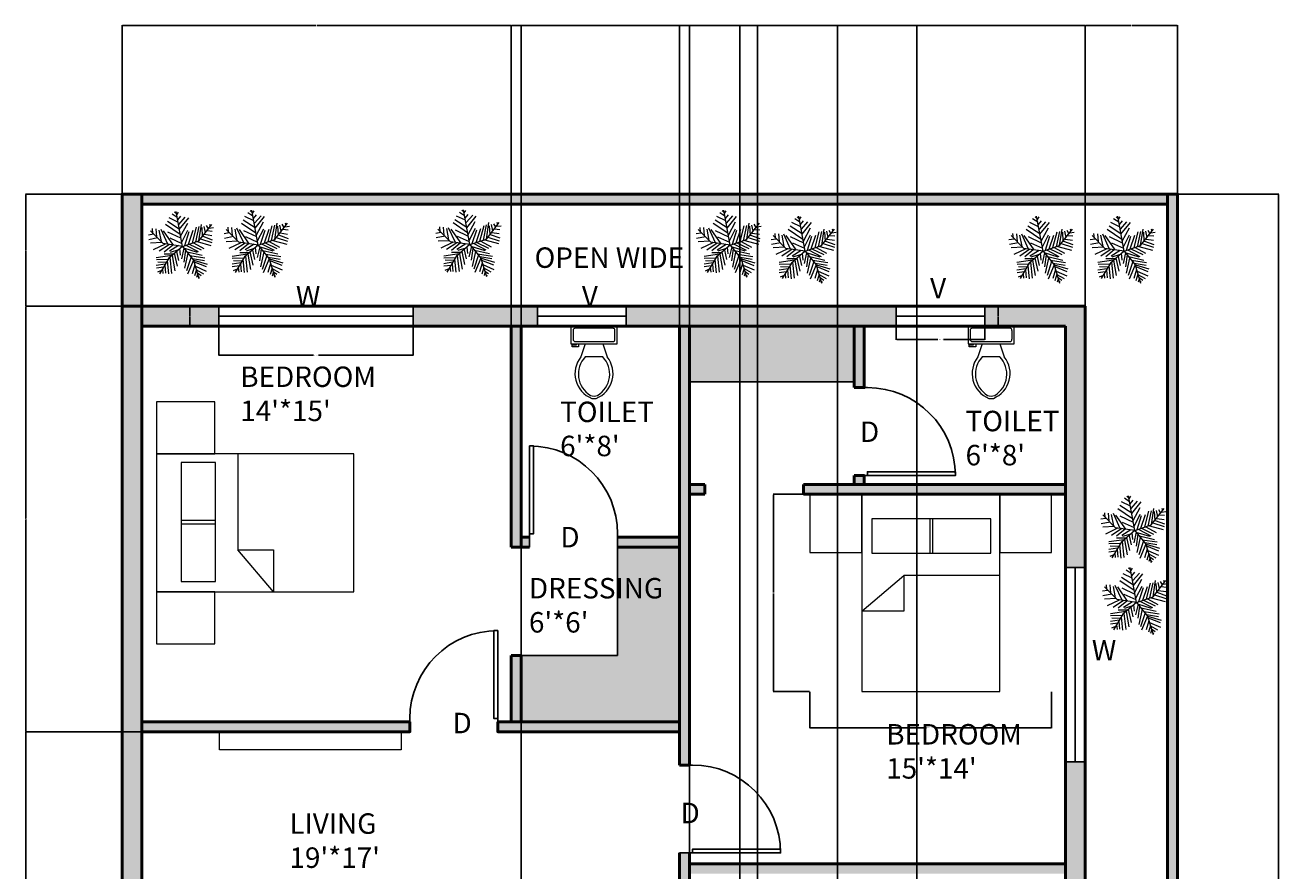
# Model space of a CAD drawing. Units: inches. Extents: x 2024 to 2594, y 643 to 1604.
# Tile 4 of 4: x 2024 to 2594, y 1219 to 1604. Entities that reach past the tile are written whole.
import ezdxf

# ---------------------------------------------------------------- set-up
doc = ezdxf.new("R2010")
doc.units = ezdxf.units.IN
for name, color, linetype, lineweight in [('A-ANNO-DIMS', 2, 'Continuous', 18), ('A-ANNO-TEXT', 7, 'Continuous', 18), ('A-AREA-IDEN', 7, 'Continuous', 25), ('A-CASE-PATT', 54, 'Continuous', 13), ('A-FLOR-CASE', 30, 'Continuous', 25), ('A-FLOR-FIXT', 8, 'Continuous', 18), ('A-WALL-PATT', 50, 'Continuous', 13), ('C-PROP', 7, 'Continuous', 35), ('DOOR', 240, 'Continuous', 25), ('FUR', 212, 'Continuous', 18), ('TREE', 102, 'Continuous', 18), ('WALL', 50, 'Continuous', 50), ('WIN', 140, 'Continuous', 25)]:
    doc.layers.add(name, color=color, linetype=linetype, lineweight=lineweight)
doc.styles.get("Standard").update_dxf_attribs({"font": 'arial.ttf'})
doc.dimstyles.get("Standard").update_dxf_attribs({"dimtxt": 0.18, "dimasz": 0.18, "dimexe": 0.18, "dimexo": 0.0625, "dimgap": 0.09, "dimtad": 0, "dimtih": 1, "dimtoh": 1, "dimdec": 4, "dimzin": 0, "dimdsep": 46, "dimtxsty": 'Standard', "dimcen": 0.09, "dimadec": 0, "dimazin": 0, "dimtfac": 1, "dimtdec": 4, "dimtofl": 0, "dimtmove": 0, "dimatfit": 3, "dimfxl": 1, "dimtolj": 1, "dimtzin": 0, "dimarcsym": 0})

# ---------------------------------------------------------------- blocks, each defined once
blk = doc.blocks.new('*U2')
for p, q in [((0, 0), (0, -6)), ((40, 0), (40, -6))]:
    blk.add_line(p, q)
blk.add_lwpolyline([(0, 0), (0, 40), (1.75, 40), (1.75, 0)], close=True)
blk.add_arc((0, 0), 40, 0, 90)
blk = doc.blocks.new('*U4')
for p, q in [((9.5, -6), (9.5, -2)), ((-10, -8.5), (-8, -8.5)), ((-10, -9.5), (-10, -8.5)), ((-7, -9.5), (-10, -9.5)), ((-8, -8.5), (-8, -8)), ((-7, -8), (-7, -9.5)), ((-4, -8), (-6, -14)), ((4, -8), (6, -14)), ((4, -14), (-4, -14))]:
    blk.add_line(p, q)
blk.add_lwpolyline([(10.5, -8), (10.5, 0), (-10.5, 0), (-10.5, -8)], close=True)
for points in [[(-9.5, -2), (-9.5, -6)], [(8.5, -1), (-8.5, -1)], [(-8.5, -7), (8.5, -7)]]:
    blk.add_lwpolyline(points)
for centre, radius, start, end in [((-8.62, -1.88), 0.884, 81.8699, 188.1301), ((8.62, -1.88), 0.884, 351.8699, 98.1301), ((-8.62, -6.12), 0.884, 171.8699, 278.1301), ((8.62, -6.12), 0.884, 261.8699, 8.1301), ((3.52, -21.58), 12.17, 141.4691, 247.9714), ((4.2, -21.82), 11.33, 136.3677, 238.9468), ((-3.52, -21.58), 12.17, 292.0284, 38.5307), ((-4.2, -21.82), 11.33, 301.053, 43.6321), ((0, -27.88), 4, 245.7318, 294.2682), ((0, -29), 4, 254.8605, 285.1395)]:
    blk.add_arc(centre, radius, start, end)
blk = doc.blocks.new('*U6')
for p, q in [((-7.288, 39.707), (-21.778, 46.673)), ((-8.737, 47.138), (-17.069, 52.711)), ((-10.186, 53.64), (-13.084, 55.962)), ((0, 0), (-10.5, 57)), ((-9.099, 51.782), (-6.563, 55.962)), ((-7.65, 43.423), (-2.578, 49.46)), ((-5.839, 35.992), (4.667, 48.067)), ((-5.114, 27.632), (10.463, 46.673)), ((-31.5, 4.5), (-52.5, 25.5)), ((-48.585, 21.131), (-49.309, 29.026)), ((-43.513, 28.561), (-42.427, 15.558)), ((-38.442, 26.239), (-34.819, 7.663)), ((-35.544, 28.097), (-24.314, 3.947)), ((-14.533, 2.09), (-30.834, 25.31)), ((-3.665, 19.273), (-27.574, 35.527)), ((-5.114, 28.097), (-24.676, 40.636)), ((-24.314, 23.917), (-2.941, 13.7)), ((-2.941, 16.486), (8.652, 37.85)), ((-1.129, 6.734), (9.014, 26.704)), ((3.942, 1.625), (11.187, 24.381)), ((10.101, 3.483), (17.708, 26.239)), ((16.259, 5.805), (23.142, 31.348)), ((22.055, 7.198), (27.489, 32.277)), ((27, 9), (48, 36)), ((27.127, 9.056), (31.112, 35.992)), ((31.836, 30.883), (32.561, 16.486)), ((35.096, 32.741), (37.27, 22.524)), ((38.719, 34.134), (41.979, 28.561)), ((40.53, 25.775), (48.862, 24.846)), ((43.791, 29.954), (51.036, 30.883)), ((44.153, 36.456), (45.239, 32.741)), ((-47.498, 19.737), (-55.83, 18.344)), ((-40.615, 13.7), (-55.105, 10.913)), ((-33.37, 6.269), (-52.207, 5.34)), ((-28.299, 3.483), (-47.86, -5.805)), ((-21.416, 3.018), (-38.079, -8.128)), ((0, 0), (-31.5, 4.5)), ((-15.982, 2.09), (-30.11, -9.521)), ((0, 0), (-22.5, -19.5)), ((-6.563, 1.161), (-21.416, -8.128)), ((-20.691, 13.7), (-1.129, 4.876)), ((0, 0), (27, 9)), ((0, 0), (18, -22.5)), ((6.478, 1.625), (26.04, -8.592)), ((11.187, 3.483), (30.749, -5.805)), ((18.07, 5.805), (35.096, -3.483)), ((24.229, 7.663), (46.688, 1.625)), ((29.662, 12.307), (48.137, 6.269)), ((33.285, 16.486), (48.862, 10.913)), ((36.183, 19.737), (48.137, 17.88)), ((-17.431, -15.094), (-42.789, -18.809)), ((-22.5, -19.5), (-37.5, -45)), ((-15.257, -12.772), (-30.11, -12.772)), ((-20.691, -18.345), (-17.793, -44.352)), ((-6.563, -5.805), (-19.967, -9.985)), ((-17.069, -15.094), (-12.721, -40.172)), ((-13.446, -11.378), (-8.737, -32.741)), ((-9.461, -8.592), (-6.201, -23.453)), ((-4.752, -3.483), (-3.665, -14.629)), ((2.493, -3.019), (-1.491, -20.202)), ((1.769, -2.555), (24.229, -9.521)), ((5.029, -6.27), (2.131, -25.775)), ((9.014, -11.378), (3.58, -35.992)), ((14.085, -16.951), (6.478, -40.172)), ((7.565, -9.056), (32.198, -14.629)), ((12.274, -15.094), (36.907, -18.809)), ((16.259, -19.738), (36.183, -22.989)), ((-28.299, -29.026), (-42.789, -31.348)), ((-24.314, -21.596), (-42.427, -22.06)), ((-30.834, -34.135), (-42.427, -35.528)), ((-34.457, -39.708), (-40.978, -42.494)), ((-26.849, -26.24), (-40.253, -25.775)), ((-32.646, -36.921), (-31.921, -44.352)), ((-29.023, -30.884), (-27.936, -43.887)), ((-25.038, -23.918), (-22.865, -45.281)), ((18.07, -22.524), (8.289, -45.745)), ((20.244, -30.419), (15.897, -44.816)), ((18, -22.5), (27, -52.5)), ((18.433, -22.524), (40.53, -29.026)), ((19.157, -25.311), (38.719, -33.206)), ((22.78, -37.85), (19.519, -48.532)), ((21.331, -32.741), (39.081, -40.636)), ((22.78, -38.314), (34.372, -44.816)), ((24.591, -45.745), (23.142, -50.854)), ((24.591, -43.423), (30.749, -47.603)), ((26.764, -49.925), (28.213, -50.854))]:
    blk.add_line(p, q)
blk = doc.blocks.new('BED-DOUBLE-WITH-NIGHTSTANDS')
for p, q in [((36.91, 86.39), (36.91, 42.72)), ((36.91, 42.72), (53.2, 42.72)), ((53.2, 23.62), (36.91, 42.72)), ((53.2, 42.72), (53.2, 23.62))]:
    blk.add_line(p, q)
for points in [[(0, 86.39), (26.45, 86.39), (26.45, 110.01), (0, 110.01)], [(0, 23.62), (89.75, 23.62), (89.75, 86.39), (0, 86.39)], [(11.14, 54.55), (26.84, 54.55), (26.84, 82.37), (11.14, 82.37)], [(11.14, 28.22), (26.84, 28.22), (26.84, 56.03), (11.14, 56.03)], [(0, 0), (26.45, 0), (26.45, 23.62), (0, 23.62)]]:
    blk.add_lwpolyline(points, close=True)
blk = doc.blocks.new('WINDOW-EXTERIOR')
blk.add_line((4.5, 0), (4.5, 88.37))
blk.add_lwpolyline([(0, 0), (9, 0), (9, 88.37), (0, 88.37)], close=True)
blk = doc.blocks.new('VENT-TOILET')
blk.add_line((0, 4.5), (40.27, 4.5))
blk.add_lwpolyline([(0, 0), (40.27, 0), (40.27, 9), (0, 9)], close=True)
blk = doc.blocks.new('*D17')
at = {"layer": 'A-ANNO-DIMS', "color": 0, "lineweight": -2, "transparency": 16777216}
for p, q in [((2112.29, 1466.87), (2112.29, 1453.5)), ((2200.66, 1466.87), (2200.66, 1453.5)), ((2112.47, 1453.68), (2155.36, 1453.68)), ((2200.48, 1453.68), (2157.59, 1453.68))]:
    blk.add_line(p, q, dxfattribs=at)
at = {"layer": 'A-ANNO-DIMS', "color": 0, "lineweight": 100, "transparency": 16777216}
for points in [[(2112.47, 1453.71), (2112.47, 1453.65), (2112.29, 1453.68)], [(2200.48, 1453.71), (2200.48, 1453.65), (2200.66, 1453.68)]]:
    blk.add_solid(points, dxfattribs=at)
at = {"layer": 'Defpoints', "color": 0, "lineweight": 100, "transparency": 16777216}
for p in [(2112.29, 1466.93), (2200.66, 1466.93), (2200.66, 1453.68)]:
    blk.add_point(p, dxfattribs=at)
at = {"layer": 'A-ANNO-DIMS', "color": 0, "transparency": 16777216, "insert": (2156.48, 1453.68), "char_height": 0.18, "attachment_point": 5}
blk.add_mtext('\\A1;WINDOW 88 TYP.', dxfattribs=at)
blk = doc.blocks.new('*D18')
at = {"layer": 'A-ANNO-DIMS', "color": 0, "lineweight": -2, "transparency": 16777216}
for p, q in [((2112.23, 1475.93), (2098.86, 1475.93)), ((2099.04, 1475.75), (2099.04, 1471.61)), ((2099.04, 1467.11), (2099.04, 1471.25)), ((2112.23, 1466.93), (2098.86, 1466.93))]:
    blk.add_line(p, q, dxfattribs=at)
at = {"layer": 'A-ANNO-DIMS', "color": 0, "lineweight": 100, "transparency": 16777216}
for points in [[(2099.01, 1475.75), (2099.07, 1475.75), (2099.04, 1475.93)], [(2099.01, 1467.11), (2099.07, 1467.11), (2099.04, 1466.93)]]:
    blk.add_solid(points, dxfattribs=at)
at = {"layer": 'Defpoints', "color": 0, "lineweight": 100, "transparency": 16777216}
for p in [(2112.29, 1475.93), (2099.04, 1466.93), (2112.29, 1466.93)]:
    blk.add_point(p, dxfattribs=at)
at = {"layer": 'A-ANNO-DIMS', "color": 0, "transparency": 16777216, "insert": (2099.04, 1471.43), "char_height": 0.18, "attachment_point": 5}
blk.add_mtext('\\A1;9 TYP.', dxfattribs=at)
blk = doc.blocks.new('*D19')
at = {"layer": 'A-ANNO-DIMS', "color": 0, "lineweight": -2, "transparency": 16777216}
for p, q in [((2381.02, 1300.62), (2381.02, 1284)), ((2491.03, 1300.62), (2491.03, 1284)), ((2381.2, 1284.18), (2434.08, 1284.18)), ((2490.85, 1284.18), (2437.96, 1284.18))]:
    blk.add_line(p, q, dxfattribs=at)
at = {"layer": 'A-ANNO-DIMS', "color": 0, "lineweight": 100, "transparency": 16777216}
for points in [[(2381.2, 1284.21), (2381.2, 1284.15), (2381.02, 1284.18)], [(2490.85, 1284.21), (2490.85, 1284.15), (2491.03, 1284.18)]]:
    blk.add_solid(points, dxfattribs=at)
at = {"layer": 'Defpoints', "color": 0, "lineweight": 100, "transparency": 16777216}
for p in [(2381.02, 1300.68), (2491.03, 1300.68), (2491.03, 1284.18)]:
    blk.add_point(p, dxfattribs=at)
at = {"layer": 'A-ANNO-DIMS', "color": 0, "transparency": 16777216, "insert": (2436.02, 1284.18), "char_height": 0.18, "attachment_point": 5}
blk.add_mtext('\\A1;BED & NIGHTSTANDS 110 TYP.', dxfattribs=at)
blk = doc.blocks.new('*D20')
at = {"layer": 'A-ANNO-DIMS', "color": 0, "lineweight": -2, "transparency": 16777216}
for p, q in [((2380.95, 1390.43), (2364.33, 1390.43)), ((2364.51, 1390.25), (2364.51, 1345.74)), ((2364.51, 1300.86), (2364.51, 1345.37)), ((2380.95, 1300.68), (2364.33, 1300.68))]:
    blk.add_line(p, q, dxfattribs=at)
at = {"layer": 'A-ANNO-DIMS', "color": 0, "lineweight": 100, "transparency": 16777216}
for points in [[(2364.48, 1390.25), (2364.54, 1390.25), (2364.51, 1390.43)], [(2364.48, 1300.86), (2364.54, 1300.86), (2364.51, 1300.68)]]:
    blk.add_solid(points, dxfattribs=at)
at = {"layer": 'Defpoints', "color": 0, "lineweight": 100, "transparency": 16777216}
for p in [(2381.02, 1390.43), (2364.51, 1300.68), (2381.02, 1300.68)]:
    blk.add_point(p, dxfattribs=at)
at = {"layer": 'A-ANNO-DIMS', "color": 0, "transparency": 16777216, "insert": (2364.51, 1345.56), "char_height": 0.18, "attachment_point": 5}
blk.add_mtext('\\A1;90 TYP.', dxfattribs=at)
blk = doc.blocks.new('*D23')
at = {"layer": 'A-ANNO-DIMS', "color": 0, "lineweight": -2, "transparency": 16777216}
for p, q in [((2420.38, 1466.87), (2420.38, 1460.71)), ((2460.65, 1466.87), (2460.65, 1460.71)), ((2420.56, 1460.89), (2439.25, 1460.89)), ((2460.47, 1460.89), (2441.78, 1460.89))]:
    blk.add_line(p, q, dxfattribs=at)
at = {"layer": 'A-ANNO-DIMS', "color": 0, "lineweight": 100, "transparency": 16777216}
for points in [[(2420.56, 1460.92), (2420.56, 1460.86), (2420.38, 1460.89)], [(2460.47, 1460.92), (2460.47, 1460.86), (2460.65, 1460.89)]]:
    blk.add_solid(points, dxfattribs=at)
at = {"layer": 'Defpoints', "color": 0, "lineweight": 100, "transparency": 16777216}
for p in [(2420.38, 1466.93), (2460.65, 1466.93), (2460.65, 1460.89)]:
    blk.add_point(p, dxfattribs=at)
at = {"layer": 'A-ANNO-DIMS', "color": 0, "transparency": 16777216, "insert": (2440.52, 1460.89), "char_height": 0.18, "attachment_point": 5}
blk.add_mtext('\\A1;BATH VENT 40 TYP.', dxfattribs=at)
blk = doc.blocks.new('*D24')
at = {"layer": 'A-ANNO-DIMS', "color": 0, "lineweight": -2, "transparency": 16777216}
for p, q in [((2460.72, 1475.93), (2466.87, 1475.93)), ((2466.69, 1475.75), (2466.69, 1471.61)), ((2466.69, 1467.11), (2466.69, 1471.25)), ((2460.72, 1466.93), (2466.87, 1466.93))]:
    blk.add_line(p, q, dxfattribs=at)
at = {"layer": 'A-ANNO-DIMS', "color": 0, "lineweight": 100, "transparency": 16777216}
for points in [[(2466.66, 1475.75), (2466.72, 1475.75), (2466.69, 1475.93)], [(2466.66, 1467.11), (2466.72, 1467.11), (2466.69, 1466.93)]]:
    blk.add_solid(points, dxfattribs=at)
at = {"layer": 'Defpoints', "color": 0, "lineweight": 100, "transparency": 16777216}
for p in [(2460.65, 1475.93), (2466.69, 1475.93), (2460.65, 1466.93)]:
    blk.add_point(p, dxfattribs=at)
at = {"layer": 'A-ANNO-DIMS', "color": 0, "transparency": 16777216, "insert": (2466.69, 1471.43), "char_height": 0.18, "attachment_point": 5}
blk.add_mtext('\\A1;9 TYP.', dxfattribs=at)
blk = doc.blocks.new('*D26')
at = {"layer": 'A-ANNO-DIMS', "color": 0, "lineweight": -2, "transparency": 16777216}
for p, q in [((2548.34, 1526.93), (2594.37, 1526.93)), ((2594.19, 1526.75), (2594.19, 1107.11)), ((2594.19, 687.11), (2594.19, 1106.75)), ((2548.34, 686.93), (2594.37, 686.93))]:
    blk.add_line(p, q, dxfattribs=at)
at = {"layer": 'A-ANNO-DIMS', "color": 0, "lineweight": 100, "transparency": 16777216}
for points in [[(2594.16, 1526.75), (2594.22, 1526.75), (2594.19, 1526.93)], [(2594.16, 687.11), (2594.22, 687.11), (2594.19, 686.93)]]:
    blk.add_solid(points, dxfattribs=at)
at = {"layer": 'Defpoints', "color": 0, "lineweight": 100, "transparency": 16777216}
for p in [(2548.27, 1526.93), (2594.19, 1526.93), (2548.27, 686.93)]:
    blk.add_point(p, dxfattribs=at)
at = {"layer": 'A-ANNO-DIMS', "color": 0, "transparency": 16777216, "insert": (2594.19, 1106.93), "char_height": 0.18, "attachment_point": 5}
blk.add_mtext('\\A1;840', dxfattribs=at)
blk = doc.blocks.new('*D27')
at = {"layer": 'A-ANNO-DIMS', "color": 0, "lineweight": -2, "transparency": 16777216}
for p, q in [((2068.27, 1475.99), (2068.27, 1603.82)), ((2068.45, 1603.64), (2156.49, 1603.64)), ((2245.09, 1603.64), (2157.05, 1603.64)), ((2245.27, 1466.99), (2245.27, 1603.82))]:
    blk.add_line(p, q, dxfattribs=at)
at = {"layer": 'A-ANNO-DIMS', "color": 0, "lineweight": 100, "transparency": 16777216}
for points in [[(2068.45, 1603.67), (2068.45, 1603.61), (2068.27, 1603.64)], [(2245.09, 1603.67), (2245.09, 1603.61), (2245.27, 1603.64)]]:
    blk.add_solid(points, dxfattribs=at)
at = {"layer": 'Defpoints', "color": 0, "lineweight": 100, "transparency": 16777216}
for p in [(2245.27, 1603.64), (2068.27, 1475.93), (2245.27, 1466.93)]:
    blk.add_point(p, dxfattribs=at)
at = {"layer": 'A-ANNO-DIMS', "color": 0, "transparency": 16777216, "insert": (2156.77, 1603.64), "char_height": 0.18, "attachment_point": 5}
blk.add_mtext('\\A1;177', dxfattribs=at)
blk = doc.blocks.new('*D28')
at = {"layer": 'A-ANNO-DIMS', "color": 0, "lineweight": -2, "transparency": 16777216}
for p, q in [((2245.27, 1466.99), (2245.27, 1603.82)), ((2245.45, 1603.64), (2283.2, 1603.64)), ((2321.59, 1603.64), (2283.85, 1603.64)), ((2321.77, 1466.99), (2321.77, 1603.82))]:
    blk.add_line(p, q, dxfattribs=at)
at = {"layer": 'A-ANNO-DIMS', "color": 0, "lineweight": 100, "transparency": 16777216}
for points in [[(2245.45, 1603.67), (2245.45, 1603.61), (2245.27, 1603.64)], [(2321.59, 1603.67), (2321.59, 1603.61), (2321.77, 1603.64)]]:
    blk.add_solid(points, dxfattribs=at)
at = {"layer": 'Defpoints', "color": 0, "lineweight": 100, "transparency": 16777216}
for p in [(2321.77, 1603.64), (2245.27, 1466.93), (2321.77, 1466.93)]:
    blk.add_point(p, dxfattribs=at)
at = {"layer": 'A-ANNO-DIMS', "color": 0, "transparency": 16777216, "insert": (2283.52, 1603.64), "char_height": 0.18, "attachment_point": 5}
blk.add_mtext('\\A1;76.5', dxfattribs=at)
blk = doc.blocks.new('*D29')
at = {"layer": 'A-ANNO-DIMS', "color": 0, "lineweight": -2, "transparency": 16777216}
for p, q in [((2321.77, 1466.99), (2321.77, 1603.82)), ((2321.95, 1603.64), (2413.64, 1603.64)), ((2506.09, 1603.64), (2414.41, 1603.64)), ((2506.27, 1475.99), (2506.27, 1603.82))]:
    blk.add_line(p, q, dxfattribs=at)
at = {"layer": 'A-ANNO-DIMS', "color": 0, "lineweight": 100, "transparency": 16777216}
for points in [[(2321.95, 1603.67), (2321.95, 1603.61), (2321.77, 1603.64)], [(2506.09, 1603.67), (2506.09, 1603.61), (2506.27, 1603.64)]]:
    blk.add_solid(points, dxfattribs=at)
at = {"layer": 'Defpoints', "color": 0, "lineweight": 100, "transparency": 16777216}
for p in [(2506.27, 1603.64), (2506.27, 1475.93), (2321.77, 1466.93)]:
    blk.add_point(p, dxfattribs=at)
at = {"layer": 'A-ANNO-DIMS', "color": 0, "transparency": 16777216, "insert": (2414.02, 1603.64), "char_height": 0.18, "attachment_point": 5}
blk.add_mtext('\\A1;184.5', dxfattribs=at)
blk = doc.blocks.new('*D30')
at = {"layer": 'A-ANNO-DIMS', "color": 0, "lineweight": -2, "transparency": 16777216}
for p, q in [((2506.27, 1475.99), (2506.27, 1603.82)), ((2506.45, 1603.64), (2527.05, 1603.64)), ((2548.09, 1603.64), (2527.49, 1603.64)), ((2548.27, 1526.99), (2548.27, 1603.82))]:
    blk.add_line(p, q, dxfattribs=at)
at = {"layer": 'A-ANNO-DIMS', "color": 0, "lineweight": 100, "transparency": 16777216}
for points in [[(2506.45, 1603.67), (2506.45, 1603.61), (2506.27, 1603.64)], [(2548.09, 1603.67), (2548.09, 1603.61), (2548.27, 1603.64)]]:
    blk.add_solid(points, dxfattribs=at)
at = {"layer": 'Defpoints', "color": 0, "lineweight": 100, "transparency": 16777216}
for p in [(2548.27, 1603.64), (2548.27, 1526.93), (2506.27, 1475.93)]:
    blk.add_point(p, dxfattribs=at)
at = {"layer": 'A-ANNO-DIMS', "color": 0, "transparency": 16777216, "insert": (2527.27, 1603.64), "char_height": 0.18, "attachment_point": 5}
blk.add_mtext('\\A1;42', dxfattribs=at)
blk = doc.blocks.new('*D34')
at = {"layer": 'A-ANNO-DIMS', "color": 0, "lineweight": -2, "transparency": 16777216}
for p, q in [((2077.21, 1282.43), (2024.29, 1282.43)), ((2024.47, 1282.25), (2024.47, 1178.36)), ((2024.47, 1074.1), (2024.47, 1177.99)), ((2077.21, 1073.92), (2024.29, 1073.92))]:
    blk.add_line(p, q, dxfattribs=at)
at = {"layer": 'A-ANNO-DIMS', "color": 0, "lineweight": 100, "transparency": 16777216}
for points in [[(2024.44, 1282.25), (2024.5, 1282.25), (2024.47, 1282.43)], [(2024.44, 1074.1), (2024.5, 1074.1), (2024.47, 1073.92)]]:
    blk.add_solid(points, dxfattribs=at)
at = {"layer": 'Defpoints', "color": 0, "lineweight": 100, "transparency": 16777216}
for p in [(2024.47, 1282.43), (2077.27, 1282.43), (2077.27, 1073.92)]:
    blk.add_point(p, dxfattribs=at)
at = {"layer": 'A-ANNO-DIMS', "color": 0, "transparency": 16777216, "insert": (2024.47, 1178.18), "char_height": 0.18, "attachment_point": 5}
blk.add_mtext('\\A1;208.5', dxfattribs=at)
blk = doc.blocks.new('*D35')
at = {"layer": 'A-ANNO-DIMS', "color": 0, "lineweight": -2, "transparency": 16777216}
for p, q in [((2068.21, 1475.93), (2024.29, 1475.93)), ((2024.47, 1475.75), (2024.47, 1379.36)), ((2024.47, 1282.61), (2024.47, 1379)), ((2077.21, 1282.43), (2024.29, 1282.43))]:
    blk.add_line(p, q, dxfattribs=at)
at = {"layer": 'A-ANNO-DIMS', "color": 0, "lineweight": 100, "transparency": 16777216}
for points in [[(2024.44, 1475.75), (2024.5, 1475.75), (2024.47, 1475.93)], [(2024.44, 1282.61), (2024.5, 1282.61), (2024.47, 1282.43)]]:
    blk.add_solid(points, dxfattribs=at)
at = {"layer": 'Defpoints', "color": 0, "lineweight": 100, "transparency": 16777216}
for p in [(2024.47, 1475.93), (2068.27, 1475.93), (2077.27, 1282.43)]:
    blk.add_point(p, dxfattribs=at)
at = {"layer": 'A-ANNO-DIMS', "color": 0, "transparency": 16777216, "insert": (2024.47, 1379.18), "char_height": 0.18, "attachment_point": 5}
blk.add_mtext('\\A1;193.5', dxfattribs=at)
blk = doc.blocks.new('*D36')
at = {"layer": 'A-ANNO-DIMS', "color": 0, "lineweight": -2, "transparency": 16777216}
for p, q in [((2068.21, 1526.93), (2024.29, 1526.93)), ((2024.47, 1526.75), (2024.47, 1501.61)), ((2024.47, 1476.11), (2024.47, 1501.25)), ((2068.21, 1475.93), (2024.29, 1475.93))]:
    blk.add_line(p, q, dxfattribs=at)
at = {"layer": 'A-ANNO-DIMS', "color": 0, "lineweight": 100, "transparency": 16777216}
for points in [[(2024.44, 1526.75), (2024.5, 1526.75), (2024.47, 1526.93)], [(2024.44, 1476.11), (2024.5, 1476.11), (2024.47, 1475.93)]]:
    blk.add_solid(points, dxfattribs=at)
at = {"layer": 'Defpoints', "color": 0, "lineweight": 100, "transparency": 16777216}
for p in [(2024.47, 1526.93), (2068.27, 1526.93), (2068.27, 1475.93)]:
    blk.add_point(p, dxfattribs=at)
at = {"layer": 'A-ANNO-DIMS', "color": 0, "transparency": 16777216, "insert": (2024.47, 1501.43), "char_height": 0.18, "attachment_point": 5}
blk.add_mtext('\\A1;51', dxfattribs=at)
blk = doc.blocks.new('*D37')
at = {"layer": 'A-ANNO-DIMS', "color": 0, "lineweight": -2, "transparency": 16777216}
for p, q in [((2326.27, 1217.99), (2326.27, 1603.82)), ((2326.45, 1603.64), (2359.59, 1603.64)), ((2393.52, 1603.64), (2360.38, 1603.64)), ((2393.7, 1214.56), (2393.7, 1603.82))]:
    blk.add_line(p, q, dxfattribs=at)
at = {"layer": 'A-ANNO-DIMS', "color": 0, "lineweight": 100, "transparency": 16777216}
for points in [[(2326.45, 1603.67), (2326.45, 1603.61), (2326.27, 1603.64)], [(2393.52, 1603.67), (2393.52, 1603.61), (2393.7, 1603.64)]]:
    blk.add_solid(points, dxfattribs=at)
at = {"layer": 'Defpoints', "color": 0, "lineweight": 100, "transparency": 16777216}
for p in [(2393.7, 1603.64), (2326.27, 1217.93), (2393.7, 1214.5)]:
    blk.add_point(p, dxfattribs=at)
at = {"layer": 'A-ANNO-DIMS', "color": 0, "transparency": 16777216, "insert": (2359.99, 1603.64), "char_height": 0.18, "attachment_point": 5}
blk.add_mtext('\\A1;67.43', dxfattribs=at)
blk = doc.blocks.new('*D38')
at = {"layer": 'A-ANNO-DIMS', "color": 0, "lineweight": -2, "transparency": 16777216}
for p, q in [((2393.7, 1214.56), (2393.7, 1603.82)), ((2393.88, 1603.64), (2411.26, 1603.64)), ((2429.57, 1603.64), (2412.19, 1603.64)), ((2429.75, 1214.56), (2429.75, 1603.82))]:
    blk.add_line(p, q, dxfattribs=at)
at = {"layer": 'A-ANNO-DIMS', "color": 0, "lineweight": 100, "transparency": 16777216}
for points in [[(2393.88, 1603.67), (2393.88, 1603.61), (2393.7, 1603.64)], [(2429.57, 1603.67), (2429.57, 1603.61), (2429.75, 1603.64)]]:
    blk.add_solid(points, dxfattribs=at)
at = {"layer": 'Defpoints', "color": 0, "lineweight": 100, "transparency": 16777216}
for p in [(2429.75, 1603.64), (2393.7, 1214.5), (2429.75, 1214.5)]:
    blk.add_point(p, dxfattribs=at)
at = {"layer": 'A-ANNO-DIMS', "color": 0, "transparency": 16777216, "insert": (2411.73, 1603.64), "char_height": 0.18, "attachment_point": 5}
blk.add_mtext('\\A1;36.046', dxfattribs=at)
blk = doc.blocks.new('*D48')
at = {"layer": 'A-ANNO-DIMS', "color": 0, "lineweight": -2, "transparency": 16777216}
for p, q in [((2249.77, 819.02), (2249.77, 1603.82)), ((2249.95, 1603.64), (2299.2, 1603.64)), ((2349.09, 1603.64), (2299.85, 1603.64)), ((2349.27, 860.99), (2349.27, 1603.82))]:
    blk.add_line(p, q, dxfattribs=at)
at = {"layer": 'A-ANNO-DIMS', "color": 0, "lineweight": 100, "transparency": 16777216}
for points in [[(2249.95, 1603.67), (2249.95, 1603.61), (2249.77, 1603.64)], [(2349.09, 1603.67), (2349.09, 1603.61), (2349.27, 1603.64)]]:
    blk.add_solid(points, dxfattribs=at)
at = {"layer": 'Defpoints', "color": 0, "lineweight": 100, "transparency": 16777216}
for p in [(2349.27, 1603.64), (2349.27, 860.93), (2249.77, 818.96)]:
    blk.add_point(p, dxfattribs=at)
at = {"layer": 'A-ANNO-DIMS', "color": 0, "transparency": 16777216, "insert": (2299.52, 1603.64), "char_height": 0.18, "attachment_point": 5}
blk.add_mtext('\\A1;99.5', dxfattribs=at)
blk = doc.blocks.new('*D51')
at = {"layer": 'A-ANNO-DIMS', "color": 0, "lineweight": -2, "transparency": 16777216}
for p, q in [((2349.27, 860.99), (2349.27, 1603.82)), ((2349.45, 1603.64), (2353.12, 1603.64)), ((2357.09, 1603.64), (2353.42, 1603.64)), ((2357.27, 860.99), (2357.27, 1603.82))]:
    blk.add_line(p, q, dxfattribs=at)
at = {"layer": 'A-ANNO-DIMS', "color": 0, "lineweight": 100, "transparency": 16777216}
for points in [[(2349.45, 1603.67), (2349.45, 1603.61), (2349.27, 1603.64)], [(2357.09, 1603.67), (2357.09, 1603.61), (2357.27, 1603.64)]]:
    blk.add_solid(points, dxfattribs=at)
at = {"layer": 'Defpoints', "color": 0, "lineweight": 100, "transparency": 16777216}
for p in [(2357.27, 1603.64), (2349.27, 860.93), (2357.27, 860.93)]:
    blk.add_point(p, dxfattribs=at)
at = {"layer": 'A-ANNO-DIMS', "color": 0, "transparency": 16777216, "insert": (2353.27, 1603.64), "char_height": 0.18, "attachment_point": 5}
blk.add_mtext('\\A1;8', dxfattribs=at)

msp = doc.modelspace()

# ---------------------------------------------------------------- hatches: boundary and pattern name
at = {"layer": 'A-CASE-PATT'}
h = msp.add_hatch(color=256, dxfattribs=at)
h.dxf.hatch_style = 1
h.paths.add_polyline_path([(2401.2727, 1466.9303), (2326.2727, 1466.9303), (2326.2727, 1441.6408), (2401.2727, 1441.6408)])
h = msp.add_hatch(color=256, dxfattribs=at)
h.dxf.hatch_style = 1
h.paths.add_polyline_path([(2321.7727, 1366.4303), (2293.6326, 1366.4303), (2293.6326, 1317.0819), (2249.7727, 1317.0819), (2249.7727, 1286.9303), (2321.7727, 1286.9303)])
at = {"layer": 'A-WALL-PATT'}
h = msp.add_hatch(color=256, dxfattribs=at)
h.dxf.hatch_style = 1
h.paths.add_polyline_path([(2543.7727, 1526.9303), (2077.2727, 1526.9303), (2077.2727, 1522.4303), (2543.7727, 1522.4303)])
h.paths.add_polyline_path([(2077.2727, 1526.9303), (2068.2727, 1526.9303), (2068.2727, 1475.9303), (2077.2727, 1475.9303)])
h.paths.add_polyline_path([(2077.2727, 1475.9303), (2068.2727, 1475.9303), (2068.2727, 686.9303), (2077.2727, 686.9303)])
h.paths.add_polyline_path([(2548.2727, 1526.9303), (2543.7727, 1526.9303), (2543.7727, 1522.4303), (2543.7727, 691.4303), (2548.2727, 691.4303)])
h.paths.add_polyline_path([(2249.7727, 1078.4303), (2199.5227, 1078.4303), (2199.5227, 1073.9303), (2245.2727, 1073.9303), (2249.7727, 1073.9217)])
h.paths.add_polyline_path([(2249.7727, 1073.9217), (2245.2727, 1073.9217), (2245.2727, 935.5102), (2249.7727, 935.5102)])
h.paths.add_polyline_path([(2326.2727, 1121.201), (2321.7727, 1121.201), (2321.7727, 1085.9303), (2326.2727, 1085.9303), (2326.2727, 1090.4303)])
h.paths.add_polyline_path([(2497.2727, 1090.4303), (2326.2727, 1090.4303), (2326.2727, 1085.9303), (2497.2727, 1085.9303)])
h.paths.add_polyline_path([(2326.2727, 1085.9303), (2321.7727, 1085.9303), (2321.7727, 989.0099), (2326.2727, 989.0099)])
h.paths.add_polyline_path([(2199.1605, 1286.9303), (2077.2727, 1286.9303), (2077.2727, 1282.4303), (2199.1605, 1282.4303)])
h.paths.add_polyline_path([(2321.7727, 1286.9303), (2239.1605, 1286.9303), (2239.1605, 1282.4303), (2321.7727, 1282.4303)])
h.paths.add_polyline_path([(2245.2727, 881.9303), (2214.9534, 881.9303), (2214.9534, 877.4303), (2245.2727, 877.4303)])
h.paths.add_polyline_path([(2118.9166, 881.9303), (2077.2727, 881.9303), (2077.2727, 877.4303), (2118.9166, 877.4303)])
h.paths.add_polyline_path([(2249.7727, 889.4074), (2246.315, 889.4074), (2245.2727, 889.4074), (2245.2727, 872.2078), (2249.7727, 872.2078)])
h.paths.add_polyline_path([(2405.0472, 941.9303), (2326.2727, 941.9303), (2326.2727, 937.4303), (2405.0472, 937.4303)])
h.paths.add_polyline_path([(2326.2727, 949.0099), (2321.7727, 949.0099), (2321.7727, 902.6727), (2326.2727, 902.6727)])
h.paths.add_polyline_path([(2326.2727, 871.366), (2321.7727, 871.366), (2321.7727, 865.4303), (2326.2727, 865.4303)])
h.paths.add_polyline_path([(2401.2727, 937.4303), (2396.7727, 937.4303), (2396.7727, 865.4303), (2401.2727, 865.4303)])
h.paths.add_polyline_path([(2497.2727, 941.9303), (2436.2168, 941.9303), (2436.2168, 937.4303), (2497.2727, 937.4303)])
h.paths.add_polyline_path([(2506.2727, 977.6959), (2497.2727, 977.6959), (2497.2727, 745.6665), (2506.2727, 745.6665)])
h.paths.add_polyline_path([(2497.2727, 754.6665), (2309.6667, 754.6665), (2309.6667, 745.6665), (2497.2727, 745.6665)])
h.paths.add_polyline_path([(2258.2092, 754.6665), (2245.2727, 754.6665), (2245.2727, 745.6665), (2258.2092, 745.6665)])
h.paths.add_polyline_path([(2249.7727, 772.853), (2248.7304, 772.853), (2245.2727, 772.853), (2245.2727, 754.6665), (2249.7727, 754.6665)])
h.paths.add_polyline_path([(2249.7727, 825.5234), (2245.2727, 825.5234), (2245.2727, 818.9558), (2248.7304, 818.9558), (2249.7727, 818.9558)])
h.paths.add_polyline_path([(2105.513, 1078.4303), (2077.2727, 1078.4303), (2077.2727, 1073.9303), (2105.513, 1073.9303)])
h.paths.add_polyline_path([(2326.2727, 1466.9303), (2321.7727, 1466.9303), (2321.7727, 1267.3126), (2326.2727, 1267.3126)])
h.paths.add_polyline_path([(2405.7727, 1466.9303), (2401.2727, 1466.9303), (2401.2727, 1438.953), (2405.7727, 1438.953)])
h.paths.add_polyline_path([(2405.7727, 1398.953), (2401.2727, 1398.953), (2401.2727, 1394.9303), (2405.7727, 1394.9303)])
h.paths.add_polyline_path([(2467.5339, 860.9303), (2467.5339, 865.4303), (2321.7727, 865.4303), (2321.7727, 860.9303)])
h.paths.add_polyline_path([(2488.7331, 865.4303), (2488.7331, 860.9303), (2497.2727, 860.9303), (2497.2727, 865.4303)])
h = msp.add_hatch(color=256, dxfattribs=at)
h.dxf.hatch_style = 1
h.paths.add_polyline_path([(2257.2361, 1475.9303), (2200.6585, 1475.9303), (2200.6585, 1466.9303), (2257.2361, 1466.9303)])
h.paths.add_polyline_path([(2112.2929, 1475.9303), (2077.2727, 1475.9303), (2077.2727, 1466.9303), (2112.2929, 1466.9303)])
h.paths.add_polyline_path([(2420.3831, 1475.9303), (2297.506, 1475.9303), (2297.506, 1466.9303), (2321.7727, 1466.9303), (2420.3831, 1466.9303)])
h.paths.add_polyline_path([(2249.7727, 1466.9303), (2245.2727, 1466.9303), (2245.2727, 1366.4303), (2249.7727, 1366.4303)])
h.paths.add_polyline_path([(2253.6326, 1370.9303), (2249.7727, 1370.9303), (2249.7727, 1366.4303), (2253.6326, 1366.4303)])
h.paths.add_polyline_path([(2321.7727, 1370.9303), (2293.6326, 1370.9303), (2293.6326, 1366.4303), (2321.7727, 1366.4303)])
h.paths.add_polyline_path([(2333.369, 1394.9303), (2326.2727, 1394.9303), (2326.2727, 1390.4303), (2333.369, 1390.4303)])
h.paths.add_polyline_path([(2506.2727, 1475.9303), (2460.6529, 1475.9303), (2460.6529, 1466.9303), (2474.0052, 1466.9303), (2497.2727, 1466.9303), (2497.2727, 1357.1459), (2506.2727, 1357.1459)])
h.paths.add_polyline_path([(2497.2727, 1394.9303), (2378.1903, 1394.9303), (2378.1903, 1390.4303), (2497.2727, 1390.4303)])
h.paths.add_polyline_path([(2506.2727, 1268.7803), (2497.2727, 1268.7803), (2497.2727, 1222.4303), (2497.2727, 1199.5194), (2506.2727, 1199.5194)])
h.paths.add_polyline_path([(2497.2727, 1222.4303), (2326.2727, 1222.4303), (2326.2727, 1217.9303), (2497.2727, 1217.9303)])
h.paths.add_polyline_path([(2326.2727, 1217.9303), (2326.2727, 1227.3126), (2321.7727, 1227.3126), (2321.7727, 1195.5957), (2326.2727, 1195.5957)])
h.paths.add_polyline_path([(2506.2727, 1111.1538), (2497.2727, 1111.1538), (2497.2727, 1085.9303), (2497.2727, 1066.0615), (2506.2727, 1066.0615)])
h = msp.add_hatch(color=256, dxfattribs=at)
h.dxf.hatch_style = 1
h.paths.add_polyline_path([(2249.7727, 1317.0819), (2245.2727, 1317.0819), (2245.2727, 1286.9303), (2249.7727, 1286.9303)])

# ---------------------------------------------------------------- linework, layer by layer
at = {"layer": 'A-FLOR-CASE'}
for p, q in [((2401.2727, 1441.6408), (2326.2727, 1441.6408)), ((2293.6326, 1366.4303), (2293.6326, 1317.0819)), ((2249.7727, 1317.0819), (2293.6326, 1317.0819))]:
    msp.add_line(p, q, dxfattribs=at)
at = {"layer": 'C-PROP'}
for p, q in [((2068.2727, 1526.9303), (2548.2727, 1526.9303)), ((2068.2727, 686.9303), (2068.2727, 1526.9303)), ((2548.2727, 1526.9303), (2548.2727, 686.9303))]:
    msp.add_line(p, q, dxfattribs=at)
msp.add_lwpolyline([(2548.2727, 686.9303), (2068.2727, 686.9303), (2068.2727, 1526.9303), (2548.2727, 1526.9303)], close=True, dxfattribs=at)
at = {"layer": 'FUR'}
msp.add_lwpolyline([(2112.5364, 1282.4303), (2195.2109, 1282.4303), (2195.2109, 1274.18), (2112.5364, 1274.18)], close=True, dxfattribs=at)
at = {"layer": 'WALL'}
for p, q in [((2077.2727, 1517.9303), (2077.2727, 1522.4303)), ((2077.2727, 1517.9303), (2077.2727, 1475.9303)), ((2077.2727, 1475.9303), (2506.2727, 1475.9303)), ((2506.2727, 1475.9303), (2506.2727, 745.6665)), ((2077.2727, 1466.9303), (2497.2727, 1466.9303)), ((2077.2727, 1466.9303), (2077.2727, 1286.9303)), ((2245.2727, 1366.4303), (2245.2727, 1466.9303)), ((2249.7727, 1466.9303), (2321.7727, 1466.9303)), ((2249.7727, 1366.4303), (2249.7727, 1466.9303)), ((2321.7727, 1466.9303), (2321.7727, 1286.9303)), ((2326.2727, 1466.9303), (2326.2727, 1282.4303)), ((2497.2727, 1466.9303), (2401.2727, 1466.9303)), ((2401.2727, 1466.9303), (2401.2727, 1438.953)), ((2405.7727, 1466.9303), (2405.7727, 1438.953)), ((2497.2727, 1466.9303), (2497.2727, 754.6665)), ((2401.2727, 1398.953), (2401.2727, 1394.9303)), ((2405.7727, 1398.953), (2405.7727, 1394.9303)), ((2333.369, 1394.9303), (2326.2727, 1394.9303)), ((2333.369, 1390.4303), (2333.369, 1394.9303)), ((2497.2727, 1394.9303), (2378.1903, 1394.9303)), ((2378.1903, 1390.4303), (2378.1903, 1394.9303)), ((2401.2727, 1394.9303), (2497.2727, 1394.9303)), ((2333.369, 1390.4303), (2326.2727, 1390.4303)), ((2497.2727, 1390.4303), (2378.1903, 1390.4303)), ((2497.2727, 1390.4303), (2497.2727, 1222.4303)), ((2253.6326, 1370.9303), (2249.7727, 1370.9303)), ((2321.7727, 1370.9303), (2293.6326, 1370.9303)), ((2249.7727, 1366.4303), (2245.2727, 1366.4303)), ((2253.6326, 1366.4303), (2249.7727, 1366.4303)), ((2321.7727, 1366.4303), (2293.6326, 1366.4303)), ((2245.2727, 1286.9303), (2245.2727, 1317.0819)), ((2245.2727, 1317.0819), (2249.7727, 1317.0819)), ((2249.7727, 1286.9303), (2249.7727, 1317.0819)), ((2077.2727, 1286.9303), (2199.1605, 1286.9303)), ((2239.1605, 1286.9303), (2321.7727, 1286.9303)), ((2077.2727, 1282.4303), (2199.1605, 1282.4303)), ((2077.2727, 1282.4303), (2077.2727, 1078.4303)), ((2239.1605, 1282.4303), (2321.7727, 1282.4303)), ((2321.7727, 1282.4303), (2321.7727, 1267.3126)), ((2326.2727, 1282.4303), (2326.2727, 1267.3126)), ((2326.2727, 1282.4303), (2326.2727, 1267.3126)), ((2321.7727, 1227.3126), (2321.7727, 1195.5957)), ((2326.2727, 1227.3126), (2326.2727, 1195.5957)), ((2326.2727, 1227.3126), (2326.2727, 1222.4303)), ((2497.2727, 1222.4303), (2326.2727, 1222.4303))]:
    msp.add_line(p, q, dxfattribs=at)
for points in [[(2077.2727, 1475.9303), (2068.2727, 1475.9303), (2068.2727, 1526.9303), (2077.2727, 1526.9303)], [(2543.7727, 1526.9303), (2077.2727, 1526.9303), (2077.2727, 1522.4303), (2543.7727, 1522.4303)], [(2543.7727, 691.4303), (2548.2727, 691.4303), (2548.2727, 1526.9303), (2543.7727, 1526.9303)], [(2068.2727, 1475.9303), (2077.2727, 1475.9303), (2077.2727, 686.9303), (2068.2727, 686.9303)], [(2321.7727, 1267.3126), (2326.2727, 1267.3126), (2326.2727, 1466.9303), (2321.7727, 1466.9303)], [(2401.2727, 1438.953), (2405.7727, 1438.953), (2405.7727, 1466.9303), (2401.2727, 1466.9303)], [(2401.2727, 1398.953), (2405.7727, 1398.953), (2405.7727, 1394.9303), (2401.2727, 1394.9303)], [(2199.1605, 1286.9303), (2077.2727, 1286.9303), (2077.2727, 1282.4303), (2199.1605, 1282.4303)], [(2239.1605, 1286.9303), (2321.7727, 1286.9303), (2321.7727, 1282.4303), (2239.1605, 1282.4303)]]:
    msp.add_lwpolyline(points, close=True, dxfattribs=at)
for points in [[(2077.2727, 1522.4303), (2543.7727, 1522.4303), (2543.7727, 691.4303), (2258.7401, 691.4303)], [(2077.2727, 881.9303), (2077.2727, 1517.9303)]]:
    msp.add_lwpolyline(points, dxfattribs=at)

# ---------------------------------------------------------------- block references
at = {"layer": 'A-FLOR-FIXT'}
for p in [(2282.9083, 1466.9303), (2463.5052, 1466.9303)]:
    msp.add_blockref('*U4', p, dxfattribs=at)
at = {"layer": 'DOOR', "xscale": -1, "rotation": 270}
for p in [(2407.2727, 1398.953), (2327.7727, 1227.3126)]:
    msp.add_blockref('*U2', p, dxfattribs=at)
at = {"layer": 'DOOR'}
msp.add_blockref('*U2', (2253.6326, 1372.4303), dxfattribs=at)
at = {"layer": 'DOOR', "xscale": -1}
msp.add_blockref('*U2', (2239.1605, 1288.4303), dxfattribs=at)
at = {"layer": 'FUR'}
msp.add_blockref('BED-DOUBLE-WITH-NIGHTSTANDS', (2083.966, 1322.486), dxfattribs=at)
at = {"layer": 'FUR', "rotation": 269.9999999999998}
msp.add_blockref('BED-DOUBLE-WITH-NIGHTSTANDS', (2381.0153, 1390.4307), dxfattribs=at)
at = {"layer": 'TREE', "xscale": 0.2775790715638129, "yscale": 0.2775790715638129, "zscale": 0.2775790715638129}
for p in [(2095.7296, 1503.196), (2130.1834, 1503.7942), (2226.4583, 1504.0026), (2344.8222, 1503.7727), (2378.9282, 1501.0309), (2487.1264, 1501.0309), (2523.9765, 1501.0309), (2528.8479, 1373.9828), (2529.6369, 1341.2698)]:
    msp.add_blockref('*U6', p, dxfattribs=at)
at = {"layer": 'WIN', "rotation": 269.9999999999998}
msp.add_blockref('WINDOW-EXTERIOR', (2112.293, 1475.93), dxfattribs=at)
at = {"layer": 'WIN'}
for name, p in [('VENT-TOILET', (2257.236, 1466.93)), ('VENT-TOILET', (2420.3829, 1466.93)), ('WINDOW-EXTERIOR', (2497.273, 1268.7804))]:
    msp.add_blockref(name, p, dxfattribs=at)

# ---------------------------------------------------------------- texts
at = {"layer": 'A-ANNO-TEXT', "char_height": 9.3008, "attachment_point": 1}
for s, insert in [('V', (2435.7518, 1488.7952)), ('W', (2147.3256, 1485.2311)), ('V', (2277.371, 1485.2311)), ('D', (2403.8776, 1423.5234)), ('D', (2267.6188, 1375.5714)), ('W', (2509.2969, 1324.1873)), ('D', (2218.5743, 1291.0483)), ('D', (2322.2714, 1250.1311))]:
    msp.add_mtext_dynamic_manual_height_columns(s, width=384.915388, gutter_width=46.5039, heights=[0], dxfattribs=dict(at, insert=insert))
at = {"layer": 'A-AREA-IDEN', "char_height": 9.30079, "attachment_point": 1}
for s, insert in [('OPEN WIDE', (2255.8777, 1502.7097)), ("BEDROOM\\P14'*15'", (2122.0295, 1448.54)), ("TOILET\\P6'*8'", (2267.5031, 1432.5652)), ("TOILET\\P6'*8'", (2451.8713, 1428.4018)), ("DRESSING\\P6'*6'", (2253.3128, 1352.3675)), ("BEDROOM\\P15'*14'", (2415.7988, 1285.9281)), ("LIVING\\P19'*17'", (2144.4029, 1245.328))]:
    msp.add_mtext_dynamic_manual_height_columns(s, width=384.915388, gutter_width=46.5039, heights=[0], dxfattribs=dict(at, insert=insert))

# ---------------------------------------------------------------- dimensions: what is measured, and where the dimension line sits
at = {"layer": 'A-ANNO-DIMS'}
for base, p1, p2, override, picture, middle in [((2245.2727, 1603.6424), (2068.2727, 1475.9303), (2245.2727, 1466.9303), {"dimdec": 0, "dimlfac": 1, "dimrnd": 0, "dimzin": 0, "dimdsep": 46, "dimlunit": 2}, '*D27', (2156.7727, 1603.6424)), ((2321.7727, 1603.6424), (2245.2727, 1466.9303), (2321.7727, 1466.9303), {"dimdec": 1, "dimlfac": 1, "dimrnd": 0, "dimzin": 0, "dimdsep": 46, "dimlunit": 2}, '*D28', (2283.5227, 1603.6424)), ((2349.2727, 1603.6424), (2249.7727, 818.9558), (2349.2727, 860.9303), {"dimdec": 1, "dimlfac": 1, "dimrnd": 0, "dimzin": 0, "dimdsep": 46, "dimlunit": 2}, '*D48', (2299.5227, 1603.6424)), ((2506.2727, 1603.6424), (2321.7727, 1466.9303), (2506.2727, 1475.9303), {"dimdec": 1, "dimlfac": 1, "dimrnd": 0, "dimzin": 0, "dimdsep": 46, "dimlunit": 2}, '*D29', (2414.0227, 1603.6424)), ((2393.7024, 1603.6424), (2326.2727, 1217.9303), (2393.7024, 1214.5024), {"dimdec": 2, "dimlfac": 1, "dimrnd": 0, "dimzin": 0, "dimdsep": 46, "dimlunit": 2}, '*D37', (2359.9876, 1603.6424)), ((2357.2727, 1603.6424), (2349.2727, 860.9303), (2357.2727, 860.9303), {"dimdec": 0, "dimlfac": 1, "dimrnd": 0, "dimzin": 0, "dimdsep": 46, "dimlunit": 2}, '*D51', (2353.2727, 1603.6424)), ((2429.7486, 1603.6424), (2393.7024, 1214.5024), (2429.7486, 1214.5024), {"dimdec": 3, "dimlfac": 1, "dimrnd": 0, "dimzin": 0, "dimdsep": 46, "dimlunit": 2}, '*D38', (2411.7255, 1603.6424)), ((2548.2727, 1603.6424), (2506.2727, 1475.9303), (2548.2727, 1526.9303), {"dimdec": 0, "dimlfac": 1, "dimrnd": 0, "dimzin": 0, "dimdsep": 46, "dimlunit": 2}, '*D30', (2527.2727, 1603.6424))]:
    dim = msp.add_linear_dim(base=base, p1=p1, p2=p2, dimstyle='Standard', override=override, dxfattribs=at)
    dim.commit()
    dim.dimension.update_dxf_attribs({"geometry": picture, "text_midpoint": middle})
for base, p1, p2, override, picture, middle in [((2024.4727, 1526.9303), (2068.2727, 1475.9303), (2068.2727, 1526.9303), {"dimdec": 0, "dimlfac": 1, "dimrnd": 0, "dimzin": 0, "dimdsep": 46, "dimlunit": 2}, '*D36', (2024.4727, 1501.4303)), ((2594.1903, 1526.9303), (2548.2727, 686.9303), (2548.2727, 1526.9303), {"dimdec": 0, "dimlfac": 1, "dimrnd": 0, "dimzin": 0, "dimdsep": 46, "dimlunit": 2}, '*D26', (2594.1903, 1106.9303)), ((2024.4727, 1475.9303), (2077.2727, 1282.4303), (2068.2727, 1475.9303), {"dimdec": 1, "dimlfac": 1, "dimrnd": 0, "dimzin": 0, "dimdsep": 46, "dimlunit": 2}, '*D35', (2024.4727, 1379.1803)), ((2024.4727, 1282.4303), (2077.2727, 1073.9217), (2077.2727, 1282.4303), {"dimdec": 1, "dimlfac": 1, "dimrnd": 0, "dimzin": 0, "dimdsep": 46, "dimlunit": 2}, '*D34', (2024.4727, 1178.176))]:
    dim = msp.add_linear_dim(base=base, p1=p1, p2=p2, angle=90, dimstyle='Standard', override=override, dxfattribs=at)
    dim.commit()
    dim.dimension.update_dxf_attribs({"geometry": picture, "text_midpoint": middle})
for base, p1, p2, angle, picture, middle in [((2099.038, 1466.9303), (2112.2929, 1475.9303), (2112.2929, 1466.9303), 270, '*D18', (2099.038, 1471.4303)), ((2466.6934, 1475.9303), (2460.6529, 1466.9303), (2460.6529, 1475.9303), 90, '*D24', (2466.6934, 1471.4303)), ((2364.514, 1300.6824), (2381.0157, 1390.4303), (2381.0157, 1300.6824), 270, '*D20', (2364.514, 1345.5563))]:
    dim = msp.add_linear_dim(base=base, p1=p1, p2=p2, angle=angle, text='<> TYP.', dimstyle='Standard', override={"dimdec": 0, "dimlfac": 1, "dimrnd": 0, "dimzin": 0, "dimdsep": 46, "dimlunit": 2}, dxfattribs=at)
    dim.commit()
    dim.dimension.update_dxf_attribs({"geometry": picture, "text_midpoint": middle})
for base, p1, p2, text, picture, middle in [((2200.6585, 1453.6754), (2112.2929, 1466.9303), (2200.6585, 1466.9303), 'WINDOW <> TYP.', '*D17', (2156.4757, 1453.6754)), ((2460.6529, 1460.8898), (2420.3831, 1466.9303), (2460.6529, 1466.9303), 'BATH VENT <> TYP.', '*D23', (2440.518, 1460.8898)), ((2491.0273, 1284.1807), (2381.0157, 1300.6824), (2491.0273, 1300.6824), 'BED & NIGHTSTANDS <> TYP.', '*D19', (2436.0215, 1284.1807))]:
    dim = msp.add_linear_dim(base=base, p1=p1, p2=p2, text=text, dimstyle='Standard', override={"dimdec": 0, "dimlfac": 1, "dimrnd": 0, "dimzin": 0, "dimdsep": 46, "dimlunit": 2}, dxfattribs=at)
    dim.commit()
    dim.dimension.update_dxf_attribs({"geometry": picture, "text_midpoint": middle})

doc.saveas('drawing.dxf')
